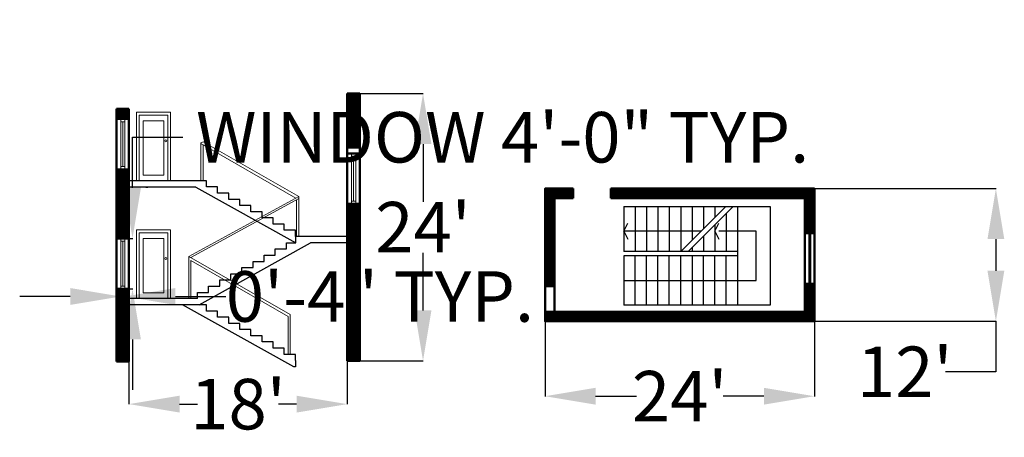
# Model space of a CAD drawing. Units: inches. Extents: x -9 to 927, y 213 to 610.
import ezdxf

# ---------------------------------------------------------------- set-up
doc = ezdxf.new("R2010")
doc.units = ezdxf.units.IN
doc.header["$MEASUREMENT"] = 0
for name, color, linetype, lineweight in [('A-ANNO-DIMS', 2, 'Continuous', 18), ('A-DOOR', 4, 'Continuous', 18), ('A-FLOR-HRAL', 6, 'Continuous', 18), ('A-FLOR-STRS', 3, 'Continuous', 25), ('A-GLAZ', 4, 'Continuous', 18), ('A-WALL', 7, 'Continuous', 50), ('A-WALL-PATT', 8, 'Continuous', 13)]:
    doc.layers.add(name, color=color, linetype=linetype, lineweight=lineweight)
doc.styles.get("Standard").update_dxf_attribs({"font": 'arial.ttf'})
doc.dimstyles.get("Standard").update_dxf_attribs({"dimtxt": 48, "dimasz": 48, "dimexe": 0.18, "dimexo": 0.0625, "dimgap": 0.09, "dimtad": 0, "dimtih": 1, "dimtoh": 1, "dimdec": 0, "dimrnd": 72, "dimzin": 0, "dimdsep": 46, "dimlunit": 3, "dimtxsty": 'Standard', "dimcen": 0.09, "dimadec": 0, "dimazin": 0, "dimtfac": 1, "dimtdec": 0, "dimtofl": 0, "dimtmove": 0, "dimatfit": 3, "dimfxl": 1, "dimtolj": 1, "dimtzin": 0, "dimarcsym": 0})

# ---------------------------------------------------------------- blocks, each defined once
blk = doc.blocks.new('*U3')
blk.add_lwpolyline([(3.1, 0), (0.1, 0), (0.1, 72), (36.1, 72), (36.1, 0), (33.1, 0)])
for points in [[(33.1, 69), (33.1, 0), (3.1, 0), (3.1, 69)], [(29.1, 6), (29.1, 63), (7.1, 63), (7.1, 6)]]:
    blk.add_lwpolyline(points, close=True)
blk.add_circle((31.1, 42), 1)
blk = doc.blocks.new('*D4')
at = {"layer": 'A-ANNO-DIMS', "color": 0, "lineweight": -2, "transparency": 16777216}
for p, q in [((314.41, 539.94), (374.62, 539.94)), ((374.44, 491.94), (374.44, 437.17)), ((374.44, 334.04), (374.44, 388.8)), ((314.41, 286.04), (374.62, 286.04))]:
    blk.add_line(p, q, dxfattribs=at)
at = {"layer": 'A-ANNO-DIMS', "color": 0, "transparency": 16777216}
for points in [[(366.44, 491.94), (382.44, 491.94), (374.44, 539.94)], [(366.44, 334.04), (382.44, 334.04), (374.44, 286.04)]]:
    blk.add_solid(points, dxfattribs=at)
at = {"layer": 'Defpoints', "color": 0, "transparency": 16777216}
for p in [(314.34, 539.94), (314.34, 286.04), (374.44, 286.04)]:
    blk.add_point(p, dxfattribs=at)
at = {"layer": 'A-ANNO-DIMS', "color": 0, "transparency": 16777216, "insert": (374.44, 412.99), "char_height": 48, "attachment_point": 5}
blk.add_mtext("\\A1;24'", dxfattribs=at)
blk = doc.blocks.new('*D5')
at = {"layer": 'A-ANNO-DIMS', "color": 0, "lineweight": -2, "transparency": 16777216}
for p, q in [((490.42, 323.58), (490.42, 252.3)), ((746.42, 323.58), (746.42, 252.3)), ((538.42, 252.48), (577.19, 252.48)), ((698.42, 252.48), (659.66, 252.48))]:
    blk.add_line(p, q, dxfattribs=at)
at = {"layer": 'A-ANNO-DIMS', "color": 0, "transparency": 16777216}
for points in [[(538.42, 260.48), (538.42, 244.48), (490.42, 252.48)], [(698.42, 260.48), (698.42, 244.48), (746.42, 252.48)]]:
    blk.add_solid(points, dxfattribs=at)
at = {"layer": 'Defpoints', "color": 0, "transparency": 16777216}
for p in [(490.42, 323.64), (746.42, 323.64), (490.42, 252.48)]:
    blk.add_point(p, dxfattribs=at)
at = {"layer": 'A-ANNO-DIMS', "color": 0, "transparency": 16777216, "insert": (618.42, 252.48), "char_height": 48, "attachment_point": 5}
blk.add_mtext("\\A1;24'", dxfattribs=at)
blk = doc.blocks.new('*D6')
at = {"layer": 'A-ANNO-DIMS', "color": 0, "lineweight": -2, "transparency": 16777216}
for p, q in [((746.49, 449.64), (919.06, 449.64)), ((918.88, 401.64), (918.88, 371.64)), ((746.49, 323.64), (919.06, 323.64)), ((918.88, 323.64), (918.88, 275.64)), ((918.88, 275.64), (870.88, 275.64))]:
    blk.add_line(p, q, dxfattribs=at)
at = {"layer": 'A-ANNO-DIMS', "color": 0, "transparency": 16777216}
for points in [[(910.88, 401.64), (926.88, 401.64), (918.88, 449.64)], [(910.88, 371.64), (926.88, 371.64), (918.88, 323.64)]]:
    blk.add_solid(points, dxfattribs=at)
at = {"layer": 'Defpoints', "color": 0, "transparency": 16777216}
for p in [(746.42, 449.64), (746.42, 323.64), (918.88, 323.64)]:
    blk.add_point(p, dxfattribs=at)
at = {"layer": 'A-ANNO-DIMS', "color": 0, "transparency": 16777216, "insert": (832.32, 275.64), "char_height": 48, "attachment_point": 5}
blk.add_mtext("\\A1;12'", dxfattribs=at)
blk = doc.blocks.new('*D7')
at = {"layer": 'A-ANNO-DIMS', "color": 0, "lineweight": -2, "transparency": 16777216}
for p, q in [((94.99, 285.34), (94.99, 244.79)), ((302.34, 285.97), (302.34, 244.79)), ((142.99, 244.97), (160.1, 244.97)), ((254.34, 244.97), (237.23, 244.97))]:
    blk.add_line(p, q, dxfattribs=at)
at = {"layer": 'A-ANNO-DIMS', "color": 0, "transparency": 16777216}
for points in [[(142.99, 252.97), (142.99, 236.97), (94.99, 244.97)], [(254.34, 252.97), (254.34, 236.97), (302.34, 244.97)]]:
    blk.add_solid(points, dxfattribs=at)
at = {"layer": 'Defpoints', "color": 0, "transparency": 16777216}
for p in [(94.99, 285.4), (302.34, 286.04), (94.99, 244.97)]:
    blk.add_point(p, dxfattribs=at)
at = {"layer": 'A-ANNO-DIMS', "color": 0, "transparency": 16777216, "insert": (198.67, 244.97), "char_height": 48, "attachment_point": 5}
blk.add_mtext("\\A1;18'", dxfattribs=at)
blk = doc.blocks.new('WIN-ELEV-1200')
for p, q in [((87.11, 402.4), (87.11, 354.4)), ((91.11, 402.4), (91.11, 354.4)), ((91.11, 402.4), (91.11, 354.4)), ((91.11, 402.4), (91.11, 354.4)), ((89.11, 399.67), (89.11, 357.13))]:
    blk.add_line(p, q)
for points in [[(87.11, 402.4), (91.11, 402.4), (91.11, 399.67), (87.11, 399.67)], [(87.11, 357.13), (91.11, 357.13), (91.11, 354.4), (87.11, 354.4)]]:
    blk.add_lwpolyline(points, close=True)
blk = doc.blocks.new('*D9')
at = {"layer": 'A-ANNO-DIMS', "color": 0, "lineweight": -2, "transparency": 16777216}
for p, q in [((98.31, 450.4), (98.31, 498.4)), ((98.31, 498.4), (146.31, 498.4)), ((91.17, 402.4), (98.49, 402.4)), ((91.17, 354.4), (98.49, 354.4)), ((98.31, 306.4), (98.31, 258.4))]:
    blk.add_line(p, q, dxfattribs=at)
at = {"layer": 'A-ANNO-DIMS', "color": 0, "transparency": 16777216}
for points in [[(90.31, 450.4), (106.31, 450.4), (98.31, 402.4)], [(90.31, 306.4), (106.31, 306.4), (98.31, 354.4)]]:
    blk.add_solid(points, dxfattribs=at)
at = {"layer": 'Defpoints', "color": 0, "transparency": 16777216}
for p in [(91.11, 402.4), (98.31, 402.4), (91.11, 354.4)]:
    blk.add_point(p, dxfattribs=at)
at = {"layer": 'A-ANNO-DIMS', "color": 0, "transparency": 16777216, "insert": (450.1, 498.4), "char_height": 48, "attachment_point": 5}
blk.add_mtext('\\A1;WINDOW 4\'-0" TYP.', dxfattribs=at)
blk = doc.blocks.new('*D10')
at = {"layer": 'A-ANNO-DIMS', "color": 0, "lineweight": -2, "transparency": 16777216}
for p, q in [((39.11, 347.2), (-8.89, 347.2)), ((87.11, 354.34), (87.11, 347.02)), ((91.11, 354.34), (91.11, 347.02)), ((139.11, 347.2), (187.11, 347.2))]:
    blk.add_line(p, q, dxfattribs=at)
at = {"layer": 'A-ANNO-DIMS', "color": 0, "transparency": 16777216}
for points in [[(39.11, 355.2), (39.11, 339.2), (87.11, 347.2)], [(139.11, 355.2), (139.11, 339.2), (91.11, 347.2)]]:
    blk.add_solid(points, dxfattribs=at)
at = {"layer": 'Defpoints', "color": 0, "transparency": 16777216}
for p in [(87.11, 354.4), (91.11, 354.4), (91.11, 347.2)]:
    blk.add_point(p, dxfattribs=at)
at = {"layer": 'A-ANNO-DIMS', "color": 0, "transparency": 16777216, "insert": (333.49, 347.2), "char_height": 48, "attachment_point": 5}
blk.add_mtext('\\A1;0\'-4" TYP.', dxfattribs=at)

msp = doc.modelspace()

# ---------------------------------------------------------------- hatches: boundary and pattern name
at = {"layer": 'A-WALL-PATT'}
h = msp.add_hatch(dxfattribs=at)
h.set_pattern_fill('ANSI31', color=256)
h.paths.add_polyline_path([(746.42, 359.2), (737.42, 359.2), (737.42, 332.64), (499.42, 332.64), (490.42, 332.64), (490.42, 323.64), (746.42, 323.64)])
h.paths.add_polyline_path([(499.42, 440.64), (517.06, 440.64), (517.06, 449.64), (490.42, 449.64), (490.42, 357.11), (499.42, 357.11)])
h.paths.add_polyline_path([(746.42, 449.64), (552.9, 449.64), (552.9, 440.64), (737.42, 440.64), (737.42, 407.24), (746.42, 407.24)])
h.paths.add_polyline_path([(314.34, 435.08), (302.34, 435.08), (302.34, 319.12), (314.34, 319.12)])
h.paths.add_polyline_path([(314.34, 539.94), (302.34, 539.94), (302.34, 488.76), (314.34, 488.76)])
h.paths.add_polyline_path([(314.34, 319.12), (302.34, 319.12), (302.34, 286.04), (314.34, 286.04)])
h = msp.add_hatch(dxfattribs=at)
h.set_pattern_fill('ANSI31', color=256)
h.paths.add_polyline_path([(94.99, 354.4), (83.22, 354.4), (83.22, 285.4), (94.99, 285.4), (94.99, 309.4), (94.99, 318.4)])
h.paths.add_polyline_path([(94.99, 439.02), (94.99, 448.02), (94.99, 467.77), (83.22, 467.77), (83.22, 402.4), (94.99, 402.4)])
h.paths.add_polyline_path([(94.99, 525.4), (83.22, 525.4), (83.22, 515.77), (94.99, 515.77)])

# ---------------------------------------------------------------- linework, layer by layer
at = {"layer": 'A-FLOR-HRAL'}
for p, q in [((163.42, 493.1), (165.42, 494.07)), ((163.42, 457.1), (163.42, 493.1)), ((253.53, 440.64), (163.42, 492.35)), ((165.42, 494.07), (256.34, 442.18)), ((165.42, 457.1), (165.42, 491.2)), ((151.77, 385.26), (256.34, 442.18)), ((153.77, 384.11), (256.34, 440.18)), ((256.34, 442.18), (256.34, 440.18)), ((256.34, 404.18), (256.34, 440.18)), ((254.34, 404.18), (254.34, 439.08)), ((151.77, 345.26), (151.77, 385.26)), ((151.77, 385.26), (248.19, 330.22)), ((153.77, 345.26), (153.77, 381.26)), ((246.19, 328.22), (153.77, 381.26)), ((246.19, 292.22), (246.19, 328.22)), ((248.19, 292.22), (248.19, 330.22))]:
    msp.add_line(p, q, dxfattribs=at)
at = {"layer": 'A-FLOR-STRS'}
for p, q in [((158.14, 457.1), (94.99, 457.1)), ((158.59, 451.1), (94.99, 451.1)), ((110.98, 451.1), (112.98, 451.1)), ((168.7, 457.1), (158.14, 457.1)), ((158.59, 451.1), (253.63, 398.18)), ((168.7, 451.22), (168.7, 457.1)), ((179.26, 451.22), (168.7, 451.22)), ((179.26, 445.34), (179.26, 451.22)), ((189.82, 445.34), (179.26, 445.34)), ((189.82, 439.46), (189.82, 445.34)), ((200.38, 439.46), (189.82, 439.46)), ((200.38, 433.58), (200.38, 439.46)), ((210.94, 433.58), (200.38, 433.58)), ((210.94, 427.7), (210.94, 433.58)), ((565.3, 432.59), (704.39, 432.59)), ((565.3, 432.59), (565.3, 389.79)), ((576.1, 432.59), (576.1, 389.79)), ((586.9, 432.59), (586.9, 389.79)), ((597.7, 432.59), (597.7, 389.79)), ((608.5, 432.59), (608.5, 389.79)), ((619.3, 432.59), (619.3, 389.79)), ((619.3, 389.79), (662.1, 432.59)), ((626.37, 389.79), (669.17, 432.59)), ((630.1, 432.59), (630.1, 400.59)), ((640.9, 432.59), (640.9, 411.39)), ((651.7, 432.59), (651.7, 422.19)), ((673.3, 432.59), (673.3, 385.79)), ((704.39, 432.59), (704.39, 385.79)), ((221.5, 427.7), (210.94, 427.7)), ((221.5, 421.82), (221.5, 427.7)), ((232.06, 421.82), (221.5, 421.82)), ((232.06, 415.94), (232.06, 421.82)), ((662.5, 425.92), (662.5, 389.79)), ((242.62, 415.94), (232.06, 415.94)), ((242.62, 410.06), (242.62, 415.94)), ((565.3, 409.19), (569.09, 416.75)), ((651.7, 409.19), (655.49, 416.75)), ((651.7, 415.12), (651.7, 389.79)), ((253.18, 410.06), (242.62, 410.06)), ((253.18, 404.18), (253.18, 410.06)), ((300.34, 404.18), (253.18, 404.18)), ((253.63, 398.18), (253.63, 404.18)), ((302.34, 404.18), (300.34, 404.18)), ((302.34, 398.18), (302.34, 404.18)), ((565.3, 409.19), (569.09, 401.63)), ((638.7, 409.19), (565.3, 409.19)), ((640.9, 404.32), (640.9, 389.79)), ((651.7, 409.19), (655.49, 401.63)), ((691.07, 409.19), (655.53, 409.19)), ((691.07, 362.39), (691.07, 409.19)), ((161.7, 339.26), (267.52, 398.18)), ((244.62, 392.3), (244.62, 398.18)), ((244.62, 398.18), (253.63, 398.18)), ((302.34, 398.18), (267.52, 398.18)), ((630.1, 393.52), (630.1, 389.79)), ((223.5, 380.54), (223.5, 386.42)), ((223.5, 386.42), (234.06, 386.42)), ((234.06, 386.42), (234.06, 392.3)), ((234.06, 392.3), (244.62, 392.3)), ((673.3, 389.79), (565.3, 389.79)), ((673.3, 385.79), (565.3, 385.79)), ((565.3, 385.79), (565.3, 338.99)), ((576.1, 338.99), (576.1, 385.79)), ((586.9, 338.99), (586.9, 385.79)), ((597.7, 338.99), (597.7, 385.79)), ((608.5, 338.99), (608.5, 385.79)), ((619.3, 338.99), (619.3, 385.79)), ((630.1, 385.79), (630.1, 338.99)), ((640.9, 338.99), (640.9, 385.79)), ((651.7, 338.99), (651.7, 385.79)), ((662.5, 338.99), (662.5, 385.79)), ((673.3, 385.79), (673.3, 338.99)), ((704.39, 385.79), (704.39, 338.99)), ((202.38, 368.78), (202.38, 374.66)), ((202.38, 374.66), (212.94, 374.66)), ((212.94, 374.66), (212.94, 380.54)), ((212.94, 380.54), (223.5, 380.54)), ((191.82, 362.9), (191.82, 368.78)), ((191.82, 368.78), (202.38, 368.78)), ((170.7, 351.14), (170.7, 357.02)), ((170.7, 357.02), (181.26, 357.02)), ((181.26, 357.02), (181.26, 362.9)), ((181.26, 362.9), (191.82, 362.9)), ((565.3, 362.39), (691.07, 362.39)), ((160.14, 345.26), (160.14, 351.14)), ((160.14, 351.14), (170.7, 351.14)), ((160.14, 345.26), (94.99, 345.26)), ((147.81, 339.26), (94.99, 339.26)), ((251.63, 280.34), (145.81, 339.26)), ((160.14, 339.26), (147.81, 339.26)), ((168.7, 339.26), (160.14, 339.26)), ((168.7, 333.38), (168.7, 339.26)), ((704.39, 338.99), (565.3, 338.99)), ((179.26, 333.38), (168.7, 333.38)), ((179.26, 327.5), (179.26, 333.38)), ((189.82, 327.5), (179.26, 327.5)), ((189.82, 321.62), (189.82, 327.5)), ((200.38, 321.62), (189.82, 321.62)), ((200.38, 315.74), (200.38, 321.62)), ((210.94, 315.74), (200.38, 315.74)), ((210.94, 309.86), (210.94, 315.74)), ((221.5, 309.86), (210.94, 309.86)), ((221.5, 303.98), (221.5, 309.86)), ((232.06, 303.98), (221.5, 303.98)), ((232.06, 298.1), (232.06, 303.98)), ((242.62, 298.1), (232.06, 298.1)), ((242.62, 292.22), (242.62, 298.1)), ((253.18, 292.22), (242.62, 292.22)), ((253.18, 286.34), (253.18, 292.22)), ((253.18, 286.34), (253.18, 280.34)), ((253.18, 280.34), (251.63, 280.34))]:
    msp.add_line(p, q, dxfattribs=at)
at = {"layer": 'A-GLAZ'}
for p, q in [((87.11, 514.05), (87.11, 467.77)), ((741.01, 407.24), (741.01, 359.2)), ((741.92, 407.24), (741.92, 359.2)), ((742.93, 407.24), (742.93, 359.2))]:
    msp.add_line(p, q, dxfattribs=at)
for points in [[(87.11, 467.77), (87.11, 468.78), (87.12, 468.78)], [(91.11, 468.78), (91.11, 467.77)]]:
    msp.add_lwpolyline(points, dxfattribs=at)
for points in [[(741.55, 407.24), (742.39, 407.24), (742.39, 406.65), (741.55, 406.65)], [(741.55, 359.79), (742.39, 359.79), (742.39, 359.2), (741.55, 359.2)]]:
    msp.add_lwpolyline(points, close=True, dxfattribs=at)
at = {"layer": 'A-WALL'}
for p, q in [((302.34, 488.76), (302.34, 539.94)), ((314.34, 539.94), (302.34, 539.94)), ((314.34, 488.76), (314.34, 539.94)), ((83.22, 525.4), (83.22, 285.4)), ((83.22, 525.4), (94.99, 525.4)), ((94.99, 525.4), (94.99, 448.02)), ((83.24, 515.77), (95, 515.77)), ((302.34, 488.76), (302.34, 286.04)), ((314.34, 488.76), (302.34, 488.76)), ((314.34, 488.76), (314.34, 286.04)), ((302.6, 483.08), (314.36, 483.08)), ((83.24, 467.77), (95, 467.77)), ((517.06, 449.64), (517.06, 440.64)), ((552.9, 449.64), (552.9, 440.64)), ((677.13, 449.64), (569.13, 449.64)), ((94.99, 448.02), (94.99, 439.02)), ((517.06, 440.64), (499.42, 440.64)), ((499.42, 440.64), (499.42, 332.64)), ((737.42, 440.64), (552.9, 440.64)), ((737.42, 332.64), (737.42, 440.64)), ((94.99, 439.02), (94.99, 318.4)), ((302.6, 435.08), (314.36, 435.08)), ((83.22, 402.4), (94.99, 402.4)), ((737.42, 407.24), (746.42, 407.24)), ((499.42, 357.11), (490.42, 357.11)), ((737.42, 359.2), (746.42, 359.2)), ((83.22, 354.4), (94.99, 354.4)), ((499.42, 332.64), (490.42, 332.64)), ((499.42, 332.64), (737.42, 332.64)), ((94.99, 318.4), (94.99, 309.4)), ((302.34, 319.12), (314.34, 319.12)), ((94.99, 309.4), (94.99, 285.4)), ((83.22, 285.4), (94.99, 285.4)), ((302.34, 286.04), (314.34, 286.04))]:
    msp.add_line(p, q, dxfattribs=at)
msp.add_lwpolyline([(517.06, 449.64), (490.42, 449.64), (490.42, 323.64), (746.42, 323.64), (746.42, 449.64), (552.9, 449.64)], dxfattribs=at)

# ---------------------------------------------------------------- block references
at = {"layer": 'A-DOOR', "xscale": 0.9046423077907308, "yscale": 0.9046423077907308, "zscale": 0.9046423077907308}
for p in [(101.88, 457.08), (101.88, 345.24)]:
    msp.add_blockref('*U3', p, dxfattribs=at)
at = {"layer": 'A-GLAZ'}
for p in [(0.01, 113.38), (219.37, 80.69), (0, 0)]:
    msp.add_blockref('WIN-ELEV-1200', p, dxfattribs=at)

# ---------------------------------------------------------------- dimensions: what is measured, and where the dimension line sits
at = {"layer": 'A-ANNO-DIMS'}
dim = msp.add_linear_dim(base=(98.31, 402.4), p1=(91.11, 354.4), p2=(91.11, 402.4), angle=90, text='WINDOW <> TYP.', dimstyle='Standard', override={"dimdec": 1, "dimlfac": 1, "dimrnd": 0, "dimzin": 1, "dimdsep": 46, "dimlunit": 4, "dimfrac": 2}, dxfattribs=at)
dim.commit()
dim.dimension.update_dxf_attribs({"geometry": '*D9', "text_midpoint": (450.1, 498.4)})
for base, p1, p2, picture, middle in [((374.44, 286.04), (314.34, 539.94), (314.34, 286.04), '*D4', (374.44, 412.99)), ((918.88, 323.64), (746.42, 449.64), (746.42, 323.64), '*D6', (832.32, 275.64))]:
    dim = msp.add_linear_dim(base=base, p1=p1, p2=p2, angle=90, dimstyle='Standard', override={"dimclrd": 0, "dimclre": 0, "dimclrt": 0}, dxfattribs=at)
    dim.commit()
    dim.dimension.update_dxf_attribs({"geometry": picture, "text_midpoint": middle})
dim = msp.add_linear_dim(base=(91.11, 347.2), p1=(87.11, 354.4), p2=(91.11, 354.4), text='<> TYP.', dimstyle='Standard', override={"dimdec": 1, "dimlfac": 1, "dimrnd": 0, "dimzin": 1, "dimdsep": 46, "dimlunit": 4, "dimfrac": 2}, dxfattribs=at)
dim.commit()
dim.dimension.update_dxf_attribs({"geometry": '*D10', "text_midpoint": (333.49, 347.2)})
for base, p1, p2, picture, middle in [((490.42, 252.48), (746.42, 323.64), (490.42, 323.64), '*D5', (618.42, 252.48)), ((94.99, 244.97), (302.34, 286.04), (94.99, 285.4), '*D7', (198.67, 244.97))]:
    dim = msp.add_linear_dim(base=base, p1=p1, p2=p2, dimstyle='Standard', override={"dimclrd": 0, "dimclre": 0, "dimclrt": 0}, dxfattribs=at)
    dim.commit()
    dim.dimension.update_dxf_attribs({"geometry": picture, "text_midpoint": middle})

doc.saveas('drawing.dxf')
